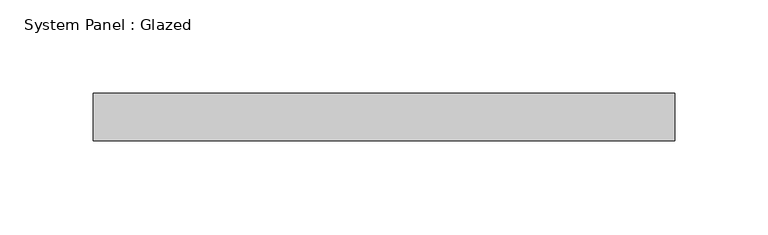
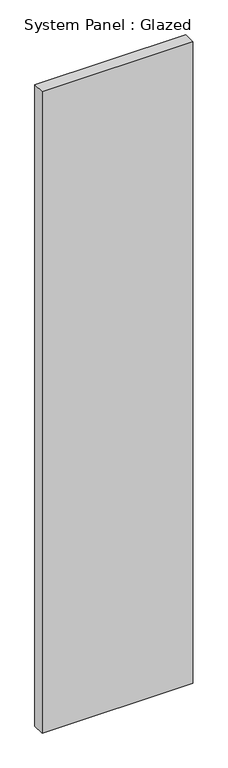
"""IFC4 building model written with IfcOpenShell, lengths in millimetres: plate geometry, System Panel : Glazed."""

from ifc_helpers import new_model, si_unit, origin, origin_with_axes, place, context, project, spatial, polyline, outline, extrude, source, transform, mapped, element, save


def system_panel_glazed_3ea5ab3e(model_context):
    return source(origin(), model_context, "Body", "SweptSolid", [
        extrude(outline(polyline([(155.575, 19.05), (-155.575, 19.05), (-155.575, 44.45), (155.575, 44.45), (155.575, 19.05)])), origin_with_axes(), (0.0, 0.0, 1.0), 1397.0),
    ])


if __name__ == "__main__":
    model = new_model("IFC4")
    model_context = context("Model", 3, world=origin())
    ifc_project = project(units=[si_unit("LENGTHUNIT", "METRE", prefix="MILLI")], contexts=[model_context])
    site = spatial("IfcSite", under=ifc_project)
    building = spatial("IfcBuilding", under=site)
    placement = place(None, origin())
    system_panel_glazed_shape = system_panel_glazed_3ea5ab3e(model_context)
    element("IfcPlate", 1, ObjectType="System Panel : Glazed", at=placement, inside=building, context=model_context, shape_type="MappedRepresentation", body=[
        mapped(system_panel_glazed_shape, transform((0.0, 0.0, 0.0), x_axis=(1.0, 0.0, 0.0), y_axis=(0.0, 1.0, 0.0), z_axis=(0.0, 0.0, 1.0))),
    ])
    save(model, "model.ifc")

# Revit data of these elements
# Type "System Panel : Glazed"
#   Construction Type Id = "GSP4R"
#   Analytic Construction = "1/8 in Pilkington single glazing"
#   Visual Light Transmittance = 0.9
#   Solar Heat Gain Coefficient = 0.86
#   Heat Transfer Coefficient (U) = 1.18115 BTU/(h·ft²·°F)
#   Define Thermal Properties by = 1
# Element 1 (IfcPlate, "System Panel : Glazed")
#   Materials on its faces: "Glass"
# Materials
#   "Glass": class "Glass", colour RGB 0 128 192, transparency 0.75, Description = "Soda Lime Glass", Cost = 0
